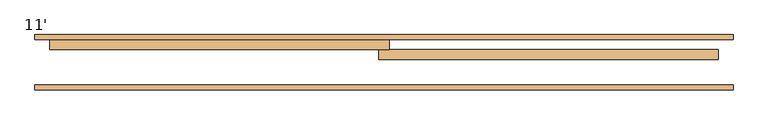
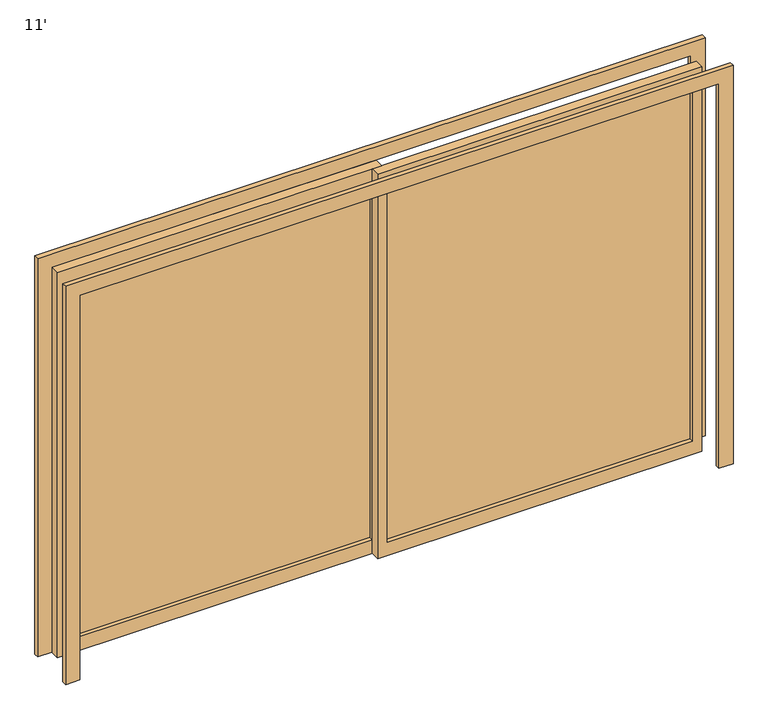
"""IFC4 building model written with IfcOpenShell, lengths in millimetres: door geometry, 11'."""

from ifc_helpers import new_model, si_unit, frame, origin, place, context, project, spatial, polyline, outline, extrude, source, transform, mapped, element, save


def door_11_423d414f(model_context):
    return source(origin(), model_context, "Body", "SweptSolid", [
        extrude(outline(polyline([(0.0, 1751.4), (2209.0, 1751.4), (2209.0, -1751.4), (0.0, -1751.4), (0.0, -1676.4), (2134.0, -1676.4), (2134.0, 1676.4), (0.0, 1676.4), (0.0, 1751.4)])), frame((0.0, 241.3, 0.0), z_axis=(0.0, 1.0, 0.0), x_axis=(0.0, 0.0, 1.0)), (0.0, 0.0, 1.0), 25.0),
        extrude(outline(polyline([(0.0, -1751.4), (0.0, -1676.4), (2134.0, -1676.4), (2134.0, 1676.4), (0.0, 1676.4), (0.0, 1751.4), (2209.0, 1751.4), (2209.0, -1751.4), (0.0, -1751.4)])), frame((0.0, -12.3, 0.0), z_axis=(0.0, 1.0, 0.0), x_axis=(0.0, 0.0, 1.0)), (0.0, 0.0, 1.0), 25.0),
        extrude(outline(polyline([(2134.0, 25.4), (2134.0, -1676.4), (0.0, -1676.4), (0.0, 25.4), (2134.0, 25.4)]), holes=[polyline([(2059.0, -24.6), (75.0, -24.6), (75.0, -1626.4), (2059.0, -1626.4), (2059.0, -24.6)])]), frame((0.0, 191.3, 0.0), z_axis=(0.0, 1.0, 0.0), x_axis=(0.0, 0.0, 1.0)), (0.0, 0.0, 1.0), 50.0),
        extrude(outline(polyline([(-1626.4, 219.475), (-24.6, 219.475), (-24.6, 213.125), (-1626.4, 213.125), (-1626.4, 219.475)])), frame((0.0, 0.0, 75.0), z_axis=(0.0, 0.0, 1.0), x_axis=(1.0, 0.0, 0.0)), (0.0, 0.0, 1.0), 1984.0),
        extrude(outline(polyline([(2134.0, -25.4), (0.0, -25.4), (0.0, 1676.4), (2134.0, 1676.4), (2134.0, -25.4)]), holes=[polyline([(2059.0, 24.6), (2059.0, 1626.4), (75.0, 1626.4), (75.0, 24.6), (2059.0, 24.6)])]), frame((0.0, 141.3, 0.0), z_axis=(0.0, 1.0, 0.0), x_axis=(0.0, 0.0, 1.0)), (0.0, 0.0, 1.0), 50.0),
        extrude(outline(polyline([(25.4, 169.475), (1626.4, 169.475), (1626.4, 163.125), (25.4, 163.125), (25.4, 169.475)])), frame((0.0, 0.0, 75.0), z_axis=(0.0, 0.0, 1.0), x_axis=(1.0, 0.0, 0.0)), (0.0, 0.0, 1.0), 1984.0),
    ])


if __name__ == "__main__":
    model = new_model("IFC4")
    model_context = context("Model", 3, world=origin())
    ifc_project = project(units=[si_unit("LENGTHUNIT", "METRE", prefix="MILLI")], contexts=[model_context])
    site = spatial("IfcSite", under=ifc_project)
    building = spatial("IfcBuilding", under=site)
    placement = place(None, origin())
    door_11_shape = door_11_423d414f(model_context)
    element("IfcDoor", 1, ObjectType="11'", at=placement, inside=building, context=model_context, shape_type="MappedRepresentation", body=[
        mapped(door_11_shape, transform((0.0, 0.0, 0.0), x_axis=(1.0, 0.0, 0.0), y_axis=(0.0, 1.0, 0.0), z_axis=(0.0, 0.0, 1.0))),
    ])
    save(model, "model.ifc")

# Revit data of these elements
# Type "11'"
#   Type Mark = "58"
#   Thickness = 0' - 1.9685"
#   Height = 7' - 0.01575"
#   Anchura de barandal = 0' - 2.95276"
#   Anchura de montante = 0' - 1.9685"
#   Proyección cubrejuntas ext. = 0' - 0.98425"
#   Proyección cubrejuntas int. = 0' - 0.98425"
#   Anchura de cubrejuntas = 0' - 2.95276"
#   Width = 11' - 0"
#   Material de puerta = Puerta - Panel
#   Function = (empty or 0)
#   Assembly Code = ""
#   Wall Closure = (empty or 0)
# Element 1 (IfcDoor, "11'")
#   Materials on its faces: "Puerta - Panel", "Cristal"
# Materials
#   "Puerta - Panel": class "Madera", colour RGB 210 159 95, transparency 0
#   "Cristal": class "Vidrio", colour RGB 0 0 255, transparency 0.75
